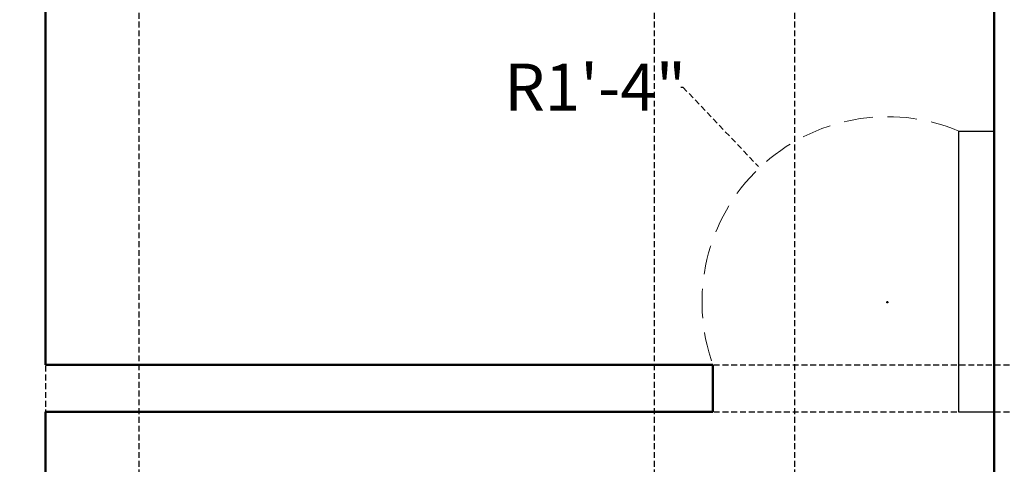
# Model space of a CAD drawing. Units: inches. Extents: x 513 to 1142, y 396 to 927.
# Tile 24 of 31: x 838 to 922, y 766 to 804. Entities that reach past the tile are written whole.
import ezdxf

# ---------------------------------------------------------------- set-up
doc = ezdxf.new("R2010")
doc.units = ezdxf.units.IN
doc.header["$MEASUREMENT"] = 0
doc.linetypes.add('DASHED', pattern=[0.75, 0.5, -0.25])
for name, color, linetype, lineweight in [('A-ANNO-DIMS', 2, 'DASHED', 18), ('A-DOOR', 4, 'Continuous', 25), ('A-DOOR-SWNG', 4, 'DASHED', 13), ('A-WALL', 7, 'Continuous', 50)]:
    doc.layers.add(name, color=color, linetype=linetype, lineweight=lineweight)
doc.styles.get("Standard").update_dxf_attribs({"font": 'arial.ttf'})
doc.dimstyles.get("Standard").update_dxf_attribs({"dimtxt": 4, "dimasz": 0.18, "dimexe": 0.18, "dimexo": 0.0625, "dimgap": 0.09, "dimtad": 0, "dimtih": 1, "dimtoh": 1, "dimdec": 0, "dimrnd": 6, "dimzin": 0, "dimdsep": 46, "dimlunit": 3, "dimtxsty": 'Standard', "dimcen": 0.09, "dimadec": 0, "dimazin": 0, "dimtfac": 1, "dimtdec": 0, "dimtofl": 0, "dimtmove": 0, "dimatfit": 3, "dimfxl": 1, "dimtolj": 1, "dimtzin": 0, "dimarcsym": 0})

# ---------------------------------------------------------------- blocks, each defined once
blk = doc.blocks.new('DOOR-LEAF-24IN')
blk.add_lwpolyline([(3, 24), (3, 0), (0, 0), (0, 24)], close=True)
blk = doc.blocks.new('*D137')
at = {"layer": 'A-ANNO-DIMS', "color": 0, "lineweight": -2, "transparency": 16777216}
for p, q in [((839.995, 770.096), (839.995, 401.578)), ((920.995, 770.067), (920.995, 401.578)), ((840.175, 401.758), (875.078, 401.758)), ((920.815, 401.758), (885.913, 401.758))]:
    blk.add_line(p, q, dxfattribs=at)
at = {"layer": 'A-ANNO-DIMS', "color": 0, "transparency": 16777216}
for points in [[(840.175, 401.788), (840.175, 401.728), (839.995, 401.758)], [(920.815, 401.788), (920.815, 401.728), (920.995, 401.758)]]:
    blk.add_solid(points, dxfattribs=at)
at = {"layer": 'Defpoints', "color": 0, "transparency": 16777216}
for p in [(839.995, 770.158), (920.995, 770.13), (920.995, 401.758)]:
    blk.add_point(p, dxfattribs=at)
at = {"layer": 'A-ANNO-DIMS', "color": 0, "transparency": 16777216, "insert": (880.495, 401.758), "char_height": 4, "attachment_point": 5}
blk.add_mtext('\\A1;6\'-9"', dxfattribs=at)
blk = doc.blocks.new('*D148')
at = {"layer": 'A-ANNO-DIMS', "color": 0, "lineweight": -2, "transparency": 16777216}
for p, q in [((921.058, 870.158), (1131.575, 870.158)), ((1131.395, 869.978), (1131.395, 824.291)), ((1131.395, 774.338), (1131.395, 820.026)), ((897.058, 774.158), (1131.575, 774.158))]:
    blk.add_line(p, q, dxfattribs=at)
at = {"layer": 'A-ANNO-DIMS', "color": 0, "transparency": 16777216}
for points in [[(1131.365, 869.978), (1131.425, 869.978), (1131.395, 870.158)], [(1131.365, 774.338), (1131.425, 774.338), (1131.395, 774.158)]]:
    blk.add_solid(points, dxfattribs=at)
at = {"layer": 'Defpoints', "color": 0, "transparency": 16777216}
for p in [(920.995, 870.158), (1131.395, 870.158), (896.995, 774.158)]:
    blk.add_point(p, dxfattribs=at)
at = {"layer": 'A-ANNO-DIMS', "color": 0, "transparency": 16777216, "insert": (1131.395, 822.158), "char_height": 4, "attachment_point": 5}
blk.add_mtext('\\A1;8\'-0"', dxfattribs=at)
blk = doc.blocks.new('*D149')
at = {"layer": 'A-ANNO-DIMS', "color": 0, "lineweight": -2, "transparency": 16777216}
for p, q in [((840.058, 770.158), (1131.575, 770.158)), ((1131.395, 769.978), (1131.395, 707.791)), ((1131.395, 641.338), (1131.395, 703.526)), ((840.058, 641.158), (1131.575, 641.158))]:
    blk.add_line(p, q, dxfattribs=at)
at = {"layer": 'A-ANNO-DIMS', "color": 0, "transparency": 16777216}
for points in [[(1131.365, 769.978), (1131.425, 769.978), (1131.395, 770.158)], [(1131.365, 641.338), (1131.425, 641.338), (1131.395, 641.158)]]:
    blk.add_solid(points, dxfattribs=at)
at = {"layer": 'Defpoints', "color": 0, "transparency": 16777216}
for p in [(839.995, 770.158), (1131.395, 770.158), (839.995, 641.158)]:
    blk.add_point(p, dxfattribs=at)
at = {"layer": 'A-ANNO-DIMS', "color": 0, "transparency": 16777216, "insert": (1131.395, 705.658), "char_height": 4, "attachment_point": 5}
blk.add_mtext('\\A1;10\'-9"', dxfattribs=at)
blk = doc.blocks.new('*D168')
at = {"layer": 'A-ANNO-DIMS', "color": 0, "lineweight": -2, "transparency": 16777216}
for p, q in [((891.995, 637.221), (891.995, 920.738)), ((892.175, 920.558), (892.777, 920.558)), ((903.815, 920.558), (903.214, 920.558)), ((903.995, 637.221), (903.995, 920.738))]:
    blk.add_line(p, q, dxfattribs=at)
at = {"layer": 'A-ANNO-DIMS', "color": 0, "transparency": 16777216}
for points in [[(892.175, 920.588), (892.175, 920.528), (891.995, 920.558)], [(903.815, 920.588), (903.815, 920.528), (903.995, 920.558)]]:
    blk.add_solid(points, dxfattribs=at)
at = {"layer": 'Defpoints', "color": 0, "transparency": 16777216}
for p in [(903.995, 920.558), (891.995, 637.158), (903.995, 637.158)]:
    blk.add_point(p, dxfattribs=at)
at = {"layer": 'A-ANNO-DIMS', "color": 0, "transparency": 16777216, "insert": (897.995, 920.558), "char_height": 4, "attachment_point": 5}
blk.add_mtext('\\A1;1\'-0"', dxfattribs=at)
blk = doc.blocks.new('*D169')
at = {"layer": 'A-ANNO-DIMS', "color": 0, "lineweight": -2, "transparency": 16777216}
for p, q in [((835.995, 774.096), (835.995, 401.578)), ((839.995, 774.096), (839.995, 401.578)), ((836.175, 401.758), (839.815, 401.758)), ((839.995, 401.758), (840.175, 401.758))]:
    blk.add_line(p, q, dxfattribs=at)
at = {"layer": 'A-ANNO-DIMS', "color": 0, "transparency": 16777216}
for points in [[(836.175, 401.788), (836.175, 401.728), (835.995, 401.758)], [(839.815, 401.788), (839.815, 401.728), (839.995, 401.758)]]:
    blk.add_solid(points, dxfattribs=at)
at = {"layer": 'Defpoints', "color": 0, "transparency": 16777216}
for p in [(835.995, 774.158), (839.995, 774.158), (839.995, 401.758)]:
    blk.add_point(p, dxfattribs=at)
at = {"layer": 'A-ANNO-DIMS', "color": 0, "transparency": 16777216, "insert": (845.582, 401.758), "char_height": 4, "attachment_point": 5}
blk.add_mtext('\\A1;0\'-4"', dxfattribs=at)
blk = doc.blocks.new('*D176')
at = {"layer": 'A-ANNO-DIMS', "color": 0, "lineweight": -2, "transparency": 16777216}
for p, q in [((847.995, 637.221), (847.995, 920.738)), ((848.175, 920.558), (864.59, 920.558)), ((891.815, 920.558), (875.4, 920.558)), ((891.995, 637.221), (891.995, 920.738))]:
    blk.add_line(p, q, dxfattribs=at)
at = {"layer": 'A-ANNO-DIMS', "color": 0, "transparency": 16777216}
for points in [[(848.175, 920.588), (848.175, 920.528), (847.995, 920.558)], [(891.815, 920.588), (891.815, 920.528), (891.995, 920.558)]]:
    blk.add_solid(points, dxfattribs=at)
at = {"layer": 'Defpoints', "color": 0, "transparency": 16777216}
for p in [(891.995, 920.558), (847.995, 637.158), (891.995, 637.158)]:
    blk.add_point(p, dxfattribs=at)
at = {"layer": 'A-ANNO-DIMS', "color": 0, "transparency": 16777216, "insert": (869.995, 920.558), "char_height": 4, "attachment_point": 5}
blk.add_mtext('\\A1;3\'-8"', dxfattribs=at)
blk = doc.blocks.new('*D192')
at = {"layer": 'A-ANNO-DIMS', "color": 0, "lineweight": -2, "transparency": 16777216}
for p, q in [((894.252, 797.88), (894.432, 797.88)), ((894.432, 797.88), (900.853, 791.128)), ((911.796, 779.528), (911.976, 779.528)), ((911.886, 779.438), (911.886, 779.618))]:
    blk.add_line(p, q, dxfattribs=at)
at = {"layer": 'A-ANNO-DIMS', "color": 0, "transparency": 16777216}
blk.add_solid([(900.875, 791.149), (900.832, 791.107), (900.977, 790.998)], dxfattribs=at)
at = {"layer": 'Defpoints', "color": 0, "transparency": 16777216}
for p in [(900.977, 790.998), (911.886, 779.528)]:
    blk.add_point(p, dxfattribs=at)
at = {"layer": 'A-ANNO-DIMS', "color": 0, "transparency": 16777216, "insert": (886.932, 797.88), "char_height": 4, "attachment_point": 5}
blk.add_mtext('\\A1;R1\'-4"', dxfattribs=at)

msp = doc.modelspace()

# ---------------------------------------------------------------- linework, layer by layer
at = {"layer": 'A-DOOR-SWNG', "ltscale": 5}
msp.add_arc((911.886, 779.528), 15.829, 67.29521, 199.82906, dxfattribs=at)
at = {"layer": 'A-WALL'}
for p, q in [((839.995, 870.158), (839.995, 774.158)), ((920.995, 710.158), (920.995, 870.158)), ((896.995, 774.158), (839.995, 774.158)), ((896.995, 770.158), (896.995, 774.158)), ((896.995, 770.158), (839.995, 770.158)), ((839.995, 770.158), (839.995, 641.158))]:
    msp.add_line(p, q, dxfattribs=at)

# ---------------------------------------------------------------- block references
at = {"layer": 'A-DOOR'}
msp.add_blockref('DOOR-LEAF-24IN', (917.995, 770.13), dxfattribs=at)

# ---------------------------------------------------------------- dimensions: what is measured, and where the dimension line sits
at = {"layer": 'A-ANNO-DIMS'}
for base, p1, p2, picture, middle in [((891.995, 920.558), (847.995, 637.158), (891.995, 637.158), '*D176', (869.995, 920.558)), ((903.995, 920.558), (891.995, 637.158), (903.995, 637.158), '*D168', (897.995, 920.558)), ((839.995, 401.758), (835.995, 774.158), (839.995, 774.158), '*D169', (845.582, 401.758)), ((920.995, 401.758), (839.995, 770.158), (920.995, 770.13), '*D137', (880.495, 401.758))]:
    dim = msp.add_linear_dim(base=base, p1=p1, p2=p2, dimstyle='Standard', override={"dimdec": 1, "dimlfac": 1, "dimrnd": 0, "dimzin": 1, "dimdsep": 46, "dimlunit": 4, "dimfrac": 2}, dxfattribs=at)
    dim.commit()
    dim.dimension.update_dxf_attribs({"geometry": picture, "text_midpoint": middle})
for base, p1, p2, picture, middle in [((1131.395, 870.158), (896.995, 774.158), (920.995, 870.158), '*D148', (1131.395, 822.158)), ((1131.395, 770.158), (839.995, 641.158), (839.995, 770.158), '*D149', (1131.395, 705.658))]:
    dim = msp.add_linear_dim(base=base, p1=p1, p2=p2, angle=90, dimstyle='Standard', override={"dimdec": 1, "dimlfac": 1, "dimrnd": 0, "dimzin": 1, "dimdsep": 46, "dimlunit": 4, "dimfrac": 2}, dxfattribs=at)
    dim.commit()
    dim.dimension.update_dxf_attribs({"geometry": picture, "text_midpoint": middle})
dim = msp.add_radius_dim(center=(911.886, 779.528), mpoint=(900.977, 790.998), dimstyle='Standard', override={"dimdec": 1, "dimlfac": 1, "dimrnd": 0, "dimzin": 1, "dimdsep": 46, "dimlunit": 4, "dimfrac": 2}, dxfattribs=at)
dim.commit()
dim.dimension.update_dxf_attribs({"geometry": '*D192', "text_midpoint": (886.932, 797.88), "dimtype": 164})

doc.saveas('drawing.dxf')
